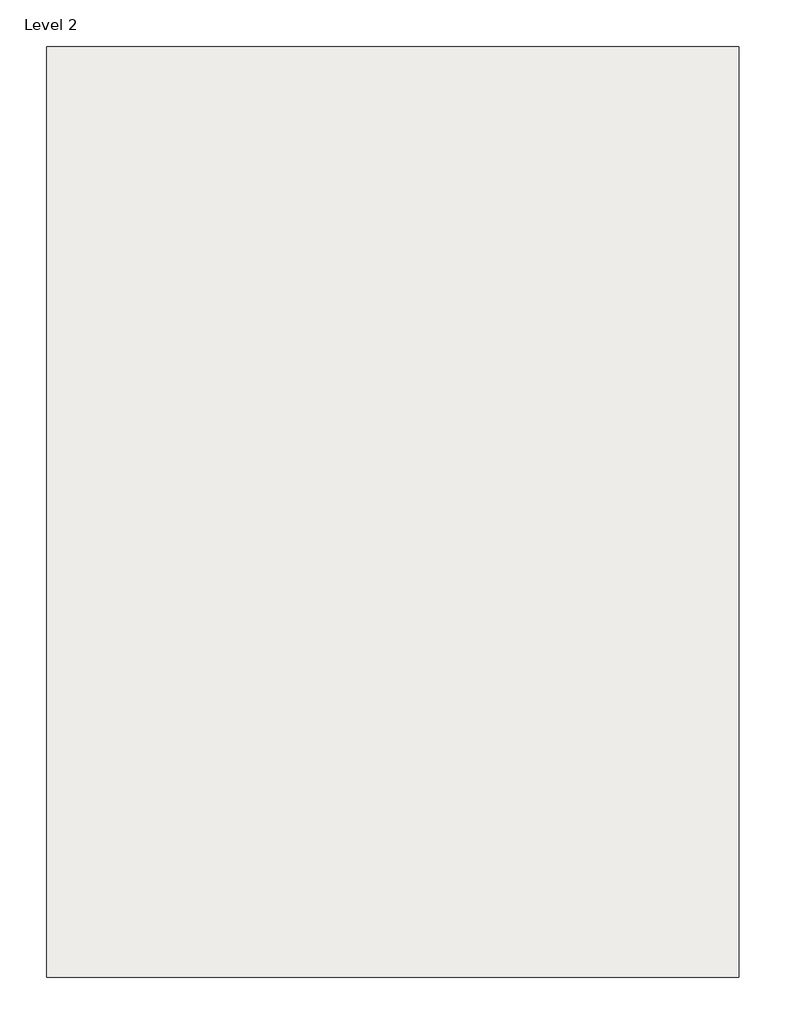
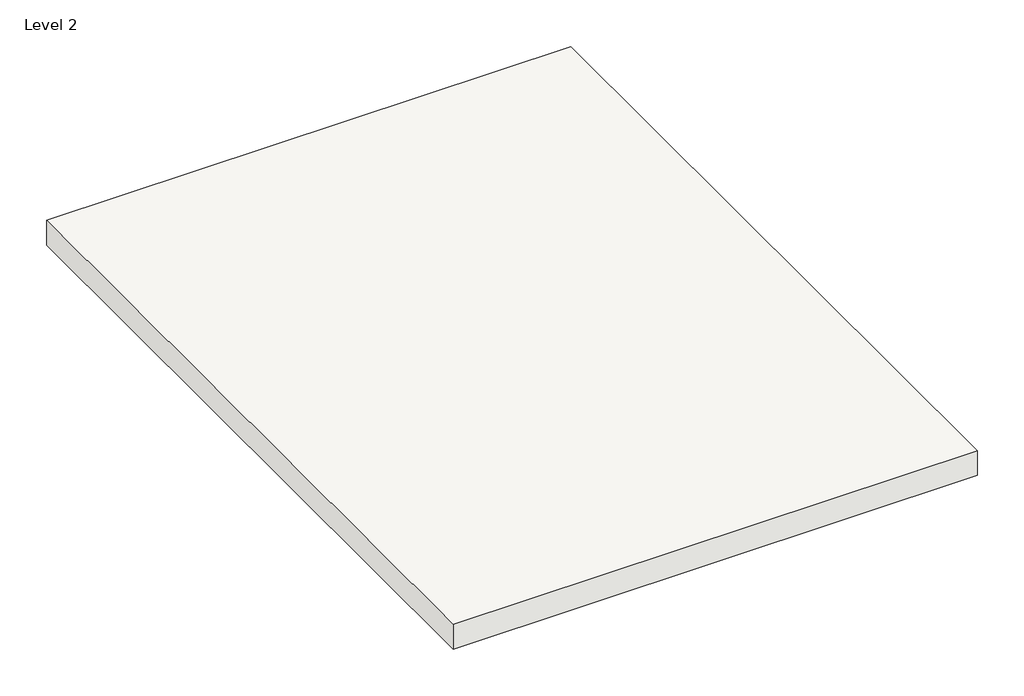
# One storey: 1 roof.
"""IFC4 building model written with IfcOpenShell, lengths in millimetres."""

from ifc_helpers import new_model, si_unit, frame, origin, place, context, project, spatial, polyline, outline, extrude, element, save

model = new_model("IFC4")

# Units and contexts
model_context = context("Model", 3, world=origin())
ifc_project = project(units=[si_unit("LENGTHUNIT", "METRE", prefix="MILLI")], contexts=[model_context])

# Site, building, storey
site = spatial("IfcSite", under=ifc_project)
building = spatial("IfcBuilding", under=site)
storey = spatial("IfcBuildingStorey", under=building, Name="Level 2", Elevation=3048.0)

# Roof
placement = place(None, origin())
element("IfcRoof", 1, ObjectType="Steel Truss - Insulation on Metal Deck - EPDM", at=placement, inside=storey, context=model_context, shape_type="SweptSolid", body=[
    extrude(outline(polyline([(-12983.1866955, 15698.6787933), (-2111.9866955, 15698.6787933), (-2111.9866955, 1093.6787933), (-12983.1866955, 1093.6787933), (-12983.1866955, 15698.6787933)])), frame((0.0, 0.0, 3048.0), z_axis=(0.0, 0.0, 1.0), x_axis=(1.0, 0.0, 0.0)), (0.0, 0.0, 1.0), 546.1),
])

save(model, "model.ifc")

# Revit data of these elements
# Type "Steel Truss - Insulation on Metal Deck - EPDM"
#   Assembly Code = "B1020"
#   Layers, outside or top first: 0' - 0 1/4" "Roofing, EPDM Membrane" (function 4); 0' - 5" "Rigid insulation" (function 3); 0' - 0 1/4" "Metal Deck" (function 1); 1' - 4" "Structure, Steel Bar Joist Layer" (function 1)
# Element 1 (IfcRoof, "Steel Truss - Insulation on Metal Deck - EPDM")
#   built-in parameter 1001705 = 11.7917 (stored number, unit not read)
#   built-in parameter 1001710 = 33615
#   Phase Created = New Construction
#   Materials on its faces: "Structure, Steel Bar Joist Layer", "Roofing, EPDM Membrane"
# Materials
#   "Roofing, EPDM Membrane": class "Generic", colour RGB 127 127 127, transparency 0, Description = "EPDM roof membrane", Cost = 0
#   "Rigid insulation": class "Generic", colour RGB 127 127 127, transparency 0, Description = "Rigid foam insulation board", Cost = 0
#   "Metal Deck": class "Metal", colour RGB 199 199 199, transparency 0, Description = "Steel, mill finish", Cost = 0
#   "Structure, Steel Bar Joist Layer": class "Metal", colour RGB 127 127 127, transparency 0, Description = "Bar joists, thermal airspace", Cost = 0
